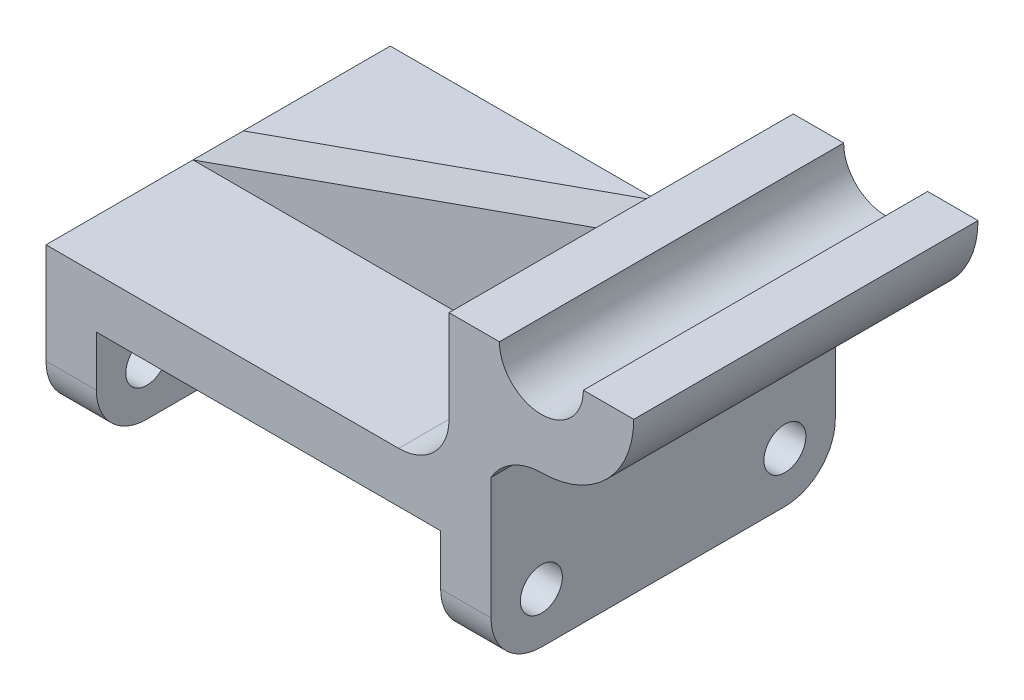
ISO-10303-21;
HEADER;
FILE_DESCRIPTION(('STEP AP214'),'2;1');
FILE_NAME('part.step','',(''),(''),'','','');
FILE_SCHEMA(('AUTOMOTIVE_DESIGN { 1 0 10303 214 1 1 1 1 }'));
ENDSEC;
DATA;
#1=APPLICATION_CONTEXT('core data for automotive mechanical design processes');
#2=APPLICATION_PROTOCOL_DEFINITION('international standard','automotive_design',2000,#1);
#3=PRODUCT_CONTEXT('',#1,'mechanical');
#4=PRODUCT('Part','Part','',(#3));
#5=PRODUCT_RELATED_PRODUCT_CATEGORY('part','',(#4));
#6=PRODUCT_DEFINITION_FORMATION('','',#4);
#7=PRODUCT_DEFINITION_CONTEXT('part definition',#1,'design');
#8=PRODUCT_DEFINITION('design','',#6,#7);
#9=PRODUCT_DEFINITION_SHAPE('','',#8);
#10=(LENGTH_UNIT() NAMED_UNIT(*) SI_UNIT(.MILLI.,.METRE.));
#11=(NAMED_UNIT(*) PLANE_ANGLE_UNIT() SI_UNIT($,.RADIAN.));
#12=(NAMED_UNIT(*) SI_UNIT($,.STERADIAN.) SOLID_ANGLE_UNIT());
#13=UNCERTAINTY_MEASURE_WITH_UNIT(LENGTH_MEASURE(1.E-05),#10,'distance_accuracy_value','');
#14=(GEOMETRIC_REPRESENTATION_CONTEXT(3) GLOBAL_UNCERTAINTY_ASSIGNED_CONTEXT((#13)) GLOBAL_UNIT_ASSIGNED_CONTEXT((#10,
#11,#12)) REPRESENTATION_CONTEXT('',''));
#15=CARTESIAN_POINT('',(0.,0.,0.));
#16=DIRECTION('',(0.,0.,1.));
#17=DIRECTION('',(1.,0.,0.));
#18=AXIS2_PLACEMENT_3D('',#15,#16,#17);
#19=CARTESIAN_POINT('',(0.,12.,0.));
#20=DIRECTION('',(0.,-1.,0.));
#21=DIRECTION('',(0.,0.,-1.));
#22=AXIS2_PLACEMENT_3D('',#19,#20,#21);
#23=PLANE('',#22);
#24=DIRECTION('',(1.,0.,0.));
#25=VECTOR('',#24,1.);
#26=CARTESIAN_POINT('',(-53.,12.,6.));
#27=LINE('',#26,#25);
#28=CARTESIAN_POINT('',(-53.,12.,6.));
#29=VERTEX_POINT('',#28);
#30=CARTESIAN_POINT('',(31.0000000000001,12.,6.));
#31=VERTEX_POINT('',#30);
#32=EDGE_CURVE('E380',#29,#31,#27,.T.);
#33=ORIENTED_EDGE('',*,*,#32,.F.);
#34=DIRECTION('',(0.,0.,1.));
#35=VECTOR('',#34,1.);
#36=CARTESIAN_POINT('',(-53.,12.,41.));
#37=LINE('',#36,#35);
#38=CARTESIAN_POINT('',(-53.,12.,41.));
#39=VERTEX_POINT('',#38);
#40=EDGE_CURVE('E368',#29,#39,#37,.T.);
#41=ORIENTED_EDGE('',*,*,#40,.T.);
#42=DIRECTION('',(1.,0.,0.));
#43=VECTOR('',#42,1.);
#44=CARTESIAN_POINT('',(-53.,12.,41.));
#45=LINE('',#44,#43);
#46=CARTESIAN_POINT('',(31.,12.,41.));
#47=VERTEX_POINT('',#46);
#48=EDGE_CURVE('E319',#39,#47,#45,.T.);
#49=ORIENTED_EDGE('',*,*,#48,.T.);
#50=DIRECTION('',(0.,0.,1.));
#51=VECTOR('',#50,1.);
#52=CARTESIAN_POINT('',(31.,12.,0.));
#53=LINE('',#52,#51);
#54=EDGE_CURVE('E230',#47,#31,#53,.F.);
#55=ORIENTED_EDGE('',*,*,#54,.T.);
#56=EDGE_LOOP('',(#33,#41,#49,#55));
#57=FACE_BOUND('',#56,.T.);
#58=ADVANCED_FACE('F39',(#57),#23,.F.);
#59=CARTESIAN_POINT('',(43.,12.,-41.));
#60=DIRECTION('',(-1.,0.,0.));
#61=DIRECTION('',(0.,0.,1.));
#62=AXIS2_PLACEMENT_3D('',#59,#60,#61);
#63=PLANE('',#62);
#64=DIRECTION('',(0.,0.,1.));
#65=VECTOR('',#64,1.);
#66=CARTESIAN_POINT('',(43.,46.,-41.));
#67=LINE('',#66,#65);
#68=CARTESIAN_POINT('',(43.,46.,6.));
#69=VERTEX_POINT('',#68);
#70=CARTESIAN_POINT('',(43.,46.,41.));
#71=VERTEX_POINT('',#70);
#72=EDGE_CURVE('E314',#69,#71,#67,.T.);
#73=ORIENTED_EDGE('',*,*,#72,.F.);
#74=DIRECTION('',(0.,1.,0.));
#75=VECTOR('',#74,1.);
#76=CARTESIAN_POINT('',(43.,46.,6.));
#77=LINE('',#76,#75);
#78=CARTESIAN_POINT('',(43.,24.,6.));
#79=VERTEX_POINT('',#78);
#80=EDGE_CURVE('E386',#79,#69,#77,.T.);
#81=ORIENTED_EDGE('',*,*,#80,.F.);
#82=DIRECTION('',(0.,0.,1.));
#83=VECTOR('',#82,1.);
#84=CARTESIAN_POINT('',(43.,24.,-41.));
#85=LINE('',#84,#83);
#86=CARTESIAN_POINT('',(43.,24.,41.));
#87=VERTEX_POINT('',#86);
#88=EDGE_CURVE('E220',#79,#87,#85,.T.);
#89=ORIENTED_EDGE('',*,*,#88,.T.);
#90=DIRECTION('',(0.,-1.,0.));
#91=VECTOR('',#90,1.);
#92=CARTESIAN_POINT('',(43.,12.,41.));
#93=LINE('',#92,#91);
#94=EDGE_CURVE('E363',#71,#87,#93,.T.);
#95=ORIENTED_EDGE('',*,*,#94,.F.);
#96=EDGE_LOOP('',(#73,#81,#89,#95));
#97=FACE_BOUND('',#96,.T.);
#98=ADVANCED_FACE('F427',(#97),#63,.T.);
#99=CARTESIAN_POINT('',(31.,24.,-41.));
#100=DIRECTION('',(0.,0.,1.));
#101=DIRECTION('',(1.,0.,0.));
#102=AXIS2_PLACEMENT_3D('',#99,#100,#101);
#103=CYLINDRICAL_SURFACE('',#102,12.);
#104=CARTESIAN_POINT('',(30.9999999999986,24.0000000000014,6.));
#105=DIRECTION('',(0.,0.,1.));
#106=DIRECTION('',(-1.,0.,0.));
#107=AXIS2_PLACEMENT_3D('',#104,#105,#106);
#108=CIRCLE('',#107,12.0000000000014);
#109=EDGE_CURVE('E510',#31,#79,#108,.T.);
#110=ORIENTED_EDGE('',*,*,#109,.F.);
#111=ORIENTED_EDGE('',*,*,#54,.F.);
#112=CARTESIAN_POINT('',(31.,24.,41.));
#113=DIRECTION('',(0.,0.,-1.));
#114=DIRECTION('',(-1.,0.,0.));
#115=AXIS2_PLACEMENT_3D('',#112,#113,#114);
#116=CIRCLE('',#115,12.);
#117=EDGE_CURVE('E235',#87,#47,#116,.T.);
#118=ORIENTED_EDGE('',*,*,#117,.F.);
#119=ORIENTED_EDGE('',*,*,#88,.F.);
#120=EDGE_LOOP('',(#110,#111,#118,#119));
#121=FACE_BOUND('',#120,.T.);
#122=ADVANCED_FACE('F440',(#121),#103,.F.);
#123=CARTESIAN_POINT('',(0.,0.,0.));
#124=DIRECTION('',(0.,-1.,0.));
#125=DIRECTION('',(0.,0.,-1.));
#126=AXIS2_PLACEMENT_3D('',#123,#124,#125);
#127=PLANE('',#126);
#128=DIRECTION('',(-1.,0.,0.));
#129=VECTOR('',#128,1.);
#130=CARTESIAN_POINT('',(-53.,0.,-41.));
#131=LINE('',#130,#129);
#132=CARTESIAN_POINT('',(41.,0.,-41.));
#133=VERTEX_POINT('',#132);
#134=CARTESIAN_POINT('',(-41.,0.,-41.));
#135=VERTEX_POINT('',#134);
#136=EDGE_CURVE('E295',#133,#135,#131,.T.);
#137=ORIENTED_EDGE('',*,*,#136,.F.);
#138=DIRECTION('',(0.,0.,1.));
#139=VECTOR('',#138,1.);
#140=CARTESIAN_POINT('',(41.,0.,41.));
#141=LINE('',#140,#139);
#142=CARTESIAN_POINT('',(41.,0.,41.));
#143=VERTEX_POINT('',#142);
#144=EDGE_CURVE('E298',#133,#143,#141,.T.);
#145=ORIENTED_EDGE('',*,*,#144,.T.);
#146=DIRECTION('',(1.,0.,0.));
#147=VECTOR('',#146,1.);
#148=CARTESIAN_POINT('',(-53.,0.,41.));
#149=LINE('',#148,#147);
#150=CARTESIAN_POINT('',(-41.,0.,41.));
#151=VERTEX_POINT('',#150);
#152=EDGE_CURVE('E307',#151,#143,#149,.T.);
#153=ORIENTED_EDGE('',*,*,#152,.F.);
#154=DIRECTION('',(0.,0.,-1.));
#155=VECTOR('',#154,1.);
#156=CARTESIAN_POINT('',(-41.,0.,-41.));
#157=LINE('',#156,#155);
#158=EDGE_CURVE('E308',#151,#135,#157,.T.);
#159=ORIENTED_EDGE('',*,*,#158,.T.);
#160=EDGE_LOOP('',(#137,#145,#153,#159));
#161=FACE_BOUND('',#160,.T.);
#162=ADVANCED_FACE('F306',(#161),#127,.T.);
#163=CARTESIAN_POINT('',(-53.,12.,-41.));
#164=VERTEX_POINT('',#163);
#165=CARTESIAN_POINT('',(-53.,12.,-6.));
#166=VERTEX_POINT('',#165);
#167=EDGE_CURVE('E367',#164,#166,#37,.T.);
#168=ORIENTED_EDGE('',*,*,#167,.T.);
#169=DIRECTION('',(1.,0.,0.));
#170=VECTOR('',#169,1.);
#171=CARTESIAN_POINT('',(-53.,12.,-6.));
#172=LINE('',#171,#170);
#173=CARTESIAN_POINT('',(31.0000000000001,12.,-6.));
#174=VERTEX_POINT('',#173);
#175=EDGE_CURVE('E480',#166,#174,#172,.T.);
#176=ORIENTED_EDGE('',*,*,#175,.T.);
#177=CARTESIAN_POINT('',(31.,12.,-41.));
#178=VERTEX_POINT('',#177);
#179=EDGE_CURVE('E226',#174,#178,#53,.F.);
#180=ORIENTED_EDGE('',*,*,#179,.T.);
#181=DIRECTION('',(-1.,0.,0.));
#182=VECTOR('',#181,1.);
#183=CARTESIAN_POINT('',(-53.,12.,-41.));
#184=LINE('',#183,#182);
#185=EDGE_CURVE('E315',#178,#164,#184,.T.);
#186=ORIENTED_EDGE('',*,*,#185,.T.);
#187=EDGE_LOOP('',(#168,#176,#180,#186));
#188=FACE_BOUND('',#187,.T.);
#189=ADVANCED_FACE('F435',(#188),#23,.F.);
#190=CARTESIAN_POINT('',(53.,12.,41.));
#191=DIRECTION('',(-1.,0.,0.));
#192=DIRECTION('',(0.,0.,1.));
#193=AXIS2_PLACEMENT_3D('',#190,#191,#192);
#194=PLANE('',#193);
#195=CARTESIAN_POINT('',(53.,-12.,29.));
#196=DIRECTION('',(1.,0.,0.));
#197=DIRECTION('',(0.,0.,-1.));
#198=AXIS2_PLACEMENT_3D('',#195,#196,#197);
#199=CIRCLE('',#198,5.);
#200=CARTESIAN_POINT('',(53.,-12.,24.));
#201=VERTEX_POINT('',#200);
#202=EDGE_CURVE('E396',#201,#201,#199,.T.);
#203=ORIENTED_EDGE('',*,*,#202,.F.);
#204=EDGE_LOOP('',(#203));
#205=FACE_BOUND('',#204,.T.);
#206=CARTESIAN_POINT('',(53.,-12.,-29.));
#207=DIRECTION('',(1.,0.,0.));
#208=DIRECTION('',(0.,0.,-1.));
#209=AXIS2_PLACEMENT_3D('',#206,#207,#208);
#210=CIRCLE('',#209,5.);
#211=CARTESIAN_POINT('',(53.,-12.,-34.));
#212=VERTEX_POINT('',#211);
#213=EDGE_CURVE('E390',#212,#212,#210,.T.);
#214=ORIENTED_EDGE('',*,*,#213,.F.);
#215=EDGE_LOOP('',(#214));
#216=FACE_BOUND('',#215,.T.);
#217=DIRECTION('',(0.,-1.,0.));
#218=VECTOR('',#217,1.);
#219=CARTESIAN_POINT('',(53.,12.,-41.));
#220=LINE('',#219,#218);
#221=CARTESIAN_POINT('',(53.,17.,-41.));
#222=VERTEX_POINT('',#221);
#223=CARTESIAN_POINT('',(53.,-12.,-41.));
#224=VERTEX_POINT('',#223);
#225=EDGE_CURVE('E207',#222,#224,#220,.T.);
#226=ORIENTED_EDGE('',*,*,#225,.F.);
#227=DIRECTION('',(0.,0.,1.));
#228=VECTOR('',#227,1.);
#229=CARTESIAN_POINT('',(53.,17.,-41.));
#230=LINE('',#229,#228);
#231=CARTESIAN_POINT('',(53.,17.,41.));
#232=VERTEX_POINT('',#231);
#233=EDGE_CURVE('E194',#222,#232,#230,.T.);
#234=ORIENTED_EDGE('',*,*,#233,.T.);
#235=DIRECTION('',(0.,-1.,0.));
#236=VECTOR('',#235,1.);
#237=CARTESIAN_POINT('',(53.,12.,41.));
#238=LINE('',#237,#236);
#239=CARTESIAN_POINT('',(53.,-12.,41.));
#240=VERTEX_POINT('',#239);
#241=EDGE_CURVE('E322',#232,#240,#238,.T.);
#242=ORIENTED_EDGE('',*,*,#241,.T.);
#243=CARTESIAN_POINT('',(53.,-12.,29.));
#244=DIRECTION('',(-1.,0.,0.));
#245=DIRECTION('',(0.,0.,1.));
#246=AXIS2_PLACEMENT_3D('',#243,#244,#245);
#247=CIRCLE('',#246,12.);
#248=CARTESIAN_POINT('',(53.,-24.,29.));
#249=VERTEX_POINT('',#248);
#250=EDGE_CURVE('E270',#240,#249,#247,.F.);
#251=ORIENTED_EDGE('',*,*,#250,.T.);
#252=DIRECTION('',(0.,0.,-1.));
#253=VECTOR('',#252,1.);
#254=CARTESIAN_POINT('',(53.,-24.,41.));
#255=LINE('',#254,#253);
#256=CARTESIAN_POINT('',(53.,-24.,-29.));
#257=VERTEX_POINT('',#256);
#258=EDGE_CURVE('E399',#249,#257,#255,.T.);
#259=ORIENTED_EDGE('',*,*,#258,.T.);
#260=CARTESIAN_POINT('',(53.,-12.,-29.));
#261=DIRECTION('',(-1.,0.,0.));
#262=DIRECTION('',(0.,0.,1.));
#263=AXIS2_PLACEMENT_3D('',#260,#261,#262);
#264=CIRCLE('',#263,12.);
#265=EDGE_CURVE('E213',#257,#224,#264,.F.);
#266=ORIENTED_EDGE('',*,*,#265,.T.);
#267=EDGE_LOOP('',(#226,#234,#242,#251,#259,#266));
#268=FACE_BOUND('',#267,.T.);
#269=ADVANCED_FACE('F214',(#205,#216,#268),#194,.F.);
#270=CARTESIAN_POINT('',(-53.,12.,-41.));
#271=DIRECTION('',(0.,0.,1.));
#272=DIRECTION('',(1.,0.,0.));
#273=AXIS2_PLACEMENT_3D('',#270,#271,#272);
#274=PLANE('',#273);
#275=DIRECTION('',(-1.,0.,0.));
#276=VECTOR('',#275,1.);
#277=CARTESIAN_POINT('',(53.,46.,-41.));
#278=LINE('',#277,#276);
#279=CARTESIAN_POINT('',(55.,46.,-41.));
#280=VERTEX_POINT('',#279);
#281=CARTESIAN_POINT('',(43.,46.,-41.));
#282=VERTEX_POINT('',#281);
#283=EDGE_CURVE('E357',#280,#282,#278,.T.);
#284=ORIENTED_EDGE('',*,*,#283,.F.);
#285=CARTESIAN_POINT('',(65.,46.,-41.));
#286=DIRECTION('',(0.,0.,-1.));
#287=DIRECTION('',(1.,0.,0.));
#288=AXIS2_PLACEMENT_3D('',#285,#286,#287);
#289=CIRCLE('',#288,10.);
#290=CARTESIAN_POINT('',(75.,46.,-41.));
#291=VERTEX_POINT('',#290);
#292=EDGE_CURVE('E202',#291,#280,#289,.T.);
#293=ORIENTED_EDGE('',*,*,#292,.F.);
#294=DIRECTION('',(-1.,0.,0.));
#295=VECTOR('',#294,1.);
#296=CARTESIAN_POINT('',(75.,46.,-41.));
#297=LINE('',#296,#295);
#298=CARTESIAN_POINT('',(87.,46.,-41.));
#299=VERTEX_POINT('',#298);
#300=EDGE_CURVE('E764',#299,#291,#297,.T.);
#301=ORIENTED_EDGE('',*,*,#300,.F.);
#302=CARTESIAN_POINT('',(65.,46.,-41.));
#303=DIRECTION('',(0.,0.,1.));
#304=DIRECTION('',(1.,0.,0.));
#305=AXIS2_PLACEMENT_3D('',#302,#303,#304);
#306=CIRCLE('',#305,22.);
#307=CARTESIAN_POINT('',(65.0760710520603,24.0001315186877,-41.));
#308=VERTEX_POINT('',#307);
#309=EDGE_CURVE('E208',#308,#299,#306,.T.);
#310=ORIENTED_EDGE('',*,*,#309,.F.);
#311=CARTESIAN_POINT('',(65.1244799033714,10.0002152123981,-41.));
#312=DIRECTION('',(0.,0.,-1.));
#313=DIRECTION('',(-1.,0.,0.));
#314=AXIS2_PLACEMENT_3D('',#311,#312,#313);
#315=CIRCLE('',#314,14.);
#316=EDGE_CURVE('E198',#222,#308,#315,.T.);
#317=ORIENTED_EDGE('',*,*,#316,.F.);
#318=ORIENTED_EDGE('',*,*,#225,.T.);
#319=DIRECTION('',(1.,0.,0.));
#320=VECTOR('',#319,1.);
#321=CARTESIAN_POINT('',(41.,-12.,-41.));
#322=LINE('',#321,#320);
#323=CARTESIAN_POINT('',(41.,-12.,-41.));
#324=VERTEX_POINT('',#323);
#325=EDGE_CURVE('E268',#224,#324,#322,.F.);
#326=ORIENTED_EDGE('',*,*,#325,.T.);
#327=DIRECTION('',(0.,1.,0.));
#328=VECTOR('',#327,1.);
#329=CARTESIAN_POINT('',(41.,0.,-41.));
#330=LINE('',#329,#328);
#331=EDGE_CURVE('E285',#324,#133,#330,.T.);
#332=ORIENTED_EDGE('',*,*,#331,.T.);
#333=ORIENTED_EDGE('',*,*,#136,.T.);
#334=DIRECTION('',(0.,-1.,0.));
#335=VECTOR('',#334,1.);
#336=CARTESIAN_POINT('',(-41.,0.,-41.));
#337=LINE('',#336,#335);
#338=CARTESIAN_POINT('',(-41.,-12.,-41.));
#339=VERTEX_POINT('',#338);
#340=EDGE_CURVE('E346',#135,#339,#337,.T.);
#341=ORIENTED_EDGE('',*,*,#340,.T.);
#342=DIRECTION('',(-1.,0.,0.));
#343=VECTOR('',#342,1.);
#344=CARTESIAN_POINT('',(-53.,-12.,-41.));
#345=LINE('',#344,#343);
#346=CARTESIAN_POINT('',(-53.,-12.,-41.));
#347=VERTEX_POINT('',#346);
#348=EDGE_CURVE('E236',#339,#347,#345,.T.);
#349=ORIENTED_EDGE('',*,*,#348,.T.);
#350=DIRECTION('',(0.,-1.,0.));
#351=VECTOR('',#350,1.);
#352=CARTESIAN_POINT('',(-53.,12.,-41.));
#353=LINE('',#352,#351);
#354=EDGE_CURVE('E216',#164,#347,#353,.T.);
#355=ORIENTED_EDGE('',*,*,#354,.F.);
#356=ORIENTED_EDGE('',*,*,#185,.F.);
#357=CARTESIAN_POINT('',(31.,24.,-41.));
#358=DIRECTION('',(0.,0.,1.));
#359=DIRECTION('',(1.,0.,0.));
#360=AXIS2_PLACEMENT_3D('',#357,#358,#359);
#361=CIRCLE('',#360,12.);
#362=CARTESIAN_POINT('',(43.,24.,-41.));
#363=VERTEX_POINT('',#362);
#364=EDGE_CURVE('E234',#178,#363,#361,.T.);
#365=ORIENTED_EDGE('',*,*,#364,.T.);
#366=DIRECTION('',(0.,-1.,0.));
#367=VECTOR('',#366,1.);
#368=CARTESIAN_POINT('',(43.,12.,-41.));
#369=LINE('',#368,#367);
#370=EDGE_CURVE('E359',#282,#363,#369,.T.);
#371=ORIENTED_EDGE('',*,*,#370,.F.);
#372=EDGE_LOOP('',(#284,#293,#301,#310,#317,#318,#326,#332,#333,#341,#349,#355,#356,#365,#371));
#373=FACE_BOUND('',#372,.T.);
#374=ADVANCED_FACE('F203',(#373),#274,.F.);
#375=CARTESIAN_POINT('',(-53.,12.,41.));
#376=DIRECTION('',(1.,0.,0.));
#377=DIRECTION('',(0.,0.,-1.));
#378=AXIS2_PLACEMENT_3D('',#375,#376,#377);
#379=PLANE('',#378);
#380=CARTESIAN_POINT('',(-53.,-12.,-29.));
#381=DIRECTION('',(-1.,0.,0.));
#382=DIRECTION('',(0.,0.,1.));
#383=AXIS2_PLACEMENT_3D('',#380,#381,#382);
#384=CIRCLE('',#383,5.);
#385=CARTESIAN_POINT('',(-53.,-12.,-24.));
#386=VERTEX_POINT('',#385);
#387=EDGE_CURVE('E256',#386,#386,#384,.T.);
#388=ORIENTED_EDGE('',*,*,#387,.F.);
#389=EDGE_LOOP('',(#388));
#390=FACE_BOUND('',#389,.T.);
#391=CARTESIAN_POINT('',(-53.,-12.,29.));
#392=DIRECTION('',(-1.,0.,0.));
#393=DIRECTION('',(0.,0.,1.));
#394=AXIS2_PLACEMENT_3D('',#391,#392,#393);
#395=CIRCLE('',#394,5.);
#396=CARTESIAN_POINT('',(-53.,-12.,34.));
#397=VERTEX_POINT('',#396);
#398=EDGE_CURVE('E303',#397,#397,#395,.T.);
#399=ORIENTED_EDGE('',*,*,#398,.F.);
#400=EDGE_LOOP('',(#399));
#401=FACE_BOUND('',#400,.T.);
#402=ORIENTED_EDGE('',*,*,#354,.T.);
#403=CARTESIAN_POINT('',(-53.,-12.,-29.));
#404=DIRECTION('',(1.,0.,0.));
#405=DIRECTION('',(0.,0.,-1.));
#406=AXIS2_PLACEMENT_3D('',#403,#404,#405);
#407=CIRCLE('',#406,12.);
#408=CARTESIAN_POINT('',(-53.,-24.,-29.));
#409=VERTEX_POINT('',#408);
#410=EDGE_CURVE('E241',#347,#409,#407,.F.);
#411=ORIENTED_EDGE('',*,*,#410,.T.);
#412=DIRECTION('',(0.,0.,1.));
#413=VECTOR('',#412,1.);
#414=CARTESIAN_POINT('',(-53.,-24.,-41.));
#415=LINE('',#414,#413);
#416=CARTESIAN_POINT('',(-53.,-24.,29.));
#417=VERTEX_POINT('',#416);
#418=EDGE_CURVE('E265',#409,#417,#415,.T.);
#419=ORIENTED_EDGE('',*,*,#418,.T.);
#420=CARTESIAN_POINT('',(-53.,-12.,29.));
#421=DIRECTION('',(1.,0.,0.));
#422=DIRECTION('',(0.,0.,-1.));
#423=AXIS2_PLACEMENT_3D('',#420,#421,#422);
#424=CIRCLE('',#423,12.);
#425=CARTESIAN_POINT('',(-53.,-12.,41.));
#426=VERTEX_POINT('',#425);
#427=EDGE_CURVE('E237',#417,#426,#424,.F.);
#428=ORIENTED_EDGE('',*,*,#427,.T.);
#429=DIRECTION('',(0.,-1.,0.));
#430=VECTOR('',#429,1.);
#431=CARTESIAN_POINT('',(-53.,12.,41.));
#432=LINE('',#431,#430);
#433=EDGE_CURVE('E224',#39,#426,#432,.T.);
#434=ORIENTED_EDGE('',*,*,#433,.F.);
#435=ORIENTED_EDGE('',*,*,#40,.F.);
#436=DIRECTION('',(0.,0.,-1.));
#437=VECTOR('',#436,1.);
#438=CARTESIAN_POINT('',(-53.,12.,6.));
#439=LINE('',#438,#437);
#440=EDGE_CURVE('E382',#29,#166,#439,.T.);
#441=ORIENTED_EDGE('',*,*,#440,.T.);
#442=ORIENTED_EDGE('',*,*,#167,.F.);
#443=EDGE_LOOP('',(#402,#411,#419,#428,#434,#435,#441,#442));
#444=FACE_BOUND('',#443,.T.);
#445=ADVANCED_FACE('F378',(#390,#401,#444),#379,.F.);
#446=CARTESIAN_POINT('',(-53.,12.,41.));
#447=DIRECTION('',(0.,0.,-1.));
#448=DIRECTION('',(-1.,0.,0.));
#449=AXIS2_PLACEMENT_3D('',#446,#447,#448);
#450=PLANE('',#449);
#451=DIRECTION('',(0.,-1.,0.));
#452=VECTOR('',#451,1.);
#453=CARTESIAN_POINT('',(41.,0.,41.));
#454=LINE('',#453,#452);
#455=CARTESIAN_POINT('',(41.,-12.,41.));
#456=VERTEX_POINT('',#455);
#457=EDGE_CURVE('E286',#143,#456,#454,.T.);
#458=ORIENTED_EDGE('',*,*,#457,.T.);
#459=DIRECTION('',(1.,0.,0.));
#460=VECTOR('',#459,1.);
#461=CARTESIAN_POINT('',(53.,-12.,41.));
#462=LINE('',#461,#460);
#463=EDGE_CURVE('E11',#456,#240,#462,.T.);
#464=ORIENTED_EDGE('',*,*,#463,.T.);
#465=ORIENTED_EDGE('',*,*,#241,.F.);
#466=CARTESIAN_POINT('',(65.1244799033714,10.0002152123981,41.));
#467=DIRECTION('',(0.,0.,-1.));
#468=DIRECTION('',(-1.,0.,0.));
#469=AXIS2_PLACEMENT_3D('',#466,#467,#468);
#470=CIRCLE('',#469,14.);
#471=CARTESIAN_POINT('',(65.0760710520603,24.0001315186877,41.));
#472=VERTEX_POINT('',#471);
#473=EDGE_CURVE('E53',#232,#472,#470,.T.);
#474=ORIENTED_EDGE('',*,*,#473,.T.);
#475=CARTESIAN_POINT('',(65.,46.,41.));
#476=DIRECTION('',(0.,0.,1.));
#477=DIRECTION('',(1.,0.,0.));
#478=AXIS2_PLACEMENT_3D('',#475,#476,#477);
#479=CIRCLE('',#478,22.);
#480=CARTESIAN_POINT('',(87.,46.,41.));
#481=VERTEX_POINT('',#480);
#482=EDGE_CURVE('E486',#472,#481,#479,.T.);
#483=ORIENTED_EDGE('',*,*,#482,.T.);
#484=DIRECTION('',(-1.,0.,0.));
#485=VECTOR('',#484,1.);
#486=CARTESIAN_POINT('',(75.,46.,41.));
#487=LINE('',#486,#485);
#488=CARTESIAN_POINT('',(75.,46.,41.));
#489=VERTEX_POINT('',#488);
#490=EDGE_CURVE('E489',#481,#489,#487,.T.);
#491=ORIENTED_EDGE('',*,*,#490,.T.);
#492=CARTESIAN_POINT('',(65.,46.,41.));
#493=DIRECTION('',(0.,0.,-1.));
#494=DIRECTION('',(1.,0.,0.));
#495=AXIS2_PLACEMENT_3D('',#492,#493,#494);
#496=CIRCLE('',#495,10.);
#497=CARTESIAN_POINT('',(55.,46.,41.));
#498=VERTEX_POINT('',#497);
#499=EDGE_CURVE('E212',#489,#498,#496,.T.);
#500=ORIENTED_EDGE('',*,*,#499,.T.);
#501=DIRECTION('',(-1.,0.,0.));
#502=VECTOR('',#501,1.);
#503=CARTESIAN_POINT('',(53.,46.,41.));
#504=LINE('',#503,#502);
#505=EDGE_CURVE('E353',#498,#71,#504,.T.);
#506=ORIENTED_EDGE('',*,*,#505,.T.);
#507=ORIENTED_EDGE('',*,*,#94,.T.);
#508=ORIENTED_EDGE('',*,*,#117,.T.);
#509=ORIENTED_EDGE('',*,*,#48,.F.);
#510=ORIENTED_EDGE('',*,*,#433,.T.);
#511=DIRECTION('',(-1.,0.,0.));
#512=VECTOR('',#511,1.);
#513=CARTESIAN_POINT('',(-41.,-12.,41.));
#514=LINE('',#513,#512);
#515=CARTESIAN_POINT('',(-41.,-12.,41.));
#516=VERTEX_POINT('',#515);
#517=EDGE_CURVE('E255',#426,#516,#514,.F.);
#518=ORIENTED_EDGE('',*,*,#517,.T.);
#519=DIRECTION('',(0.,1.,0.));
#520=VECTOR('',#519,1.);
#521=CARTESIAN_POINT('',(-41.,0.,41.));
#522=LINE('',#521,#520);
#523=EDGE_CURVE('E345',#516,#151,#522,.T.);
#524=ORIENTED_EDGE('',*,*,#523,.T.);
#525=ORIENTED_EDGE('',*,*,#152,.T.);
#526=EDGE_LOOP('',(#458,#464,#465,#474,#483,#491,#500,#506,#507,#508,#509,#510,#518,#524,#525));
#527=FACE_BOUND('',#526,.T.);
#528=ADVANCED_FACE('F330',(#527),#450,.F.);
#529=DIRECTION('',(0.,1.,0.));
#530=VECTOR('',#529,1.);
#531=CARTESIAN_POINT('',(43.,46.,-6.));
#532=LINE('',#531,#530);
#533=CARTESIAN_POINT('',(43.,24.,-6.));
#534=VERTEX_POINT('',#533);
#535=CARTESIAN_POINT('',(43.,46.,-6.));
#536=VERTEX_POINT('',#535);
#537=EDGE_CURVE('E65',#534,#536,#532,.T.);
#538=ORIENTED_EDGE('',*,*,#537,.T.);
#539=EDGE_CURVE('E309',#282,#536,#67,.T.);
#540=ORIENTED_EDGE('',*,*,#539,.F.);
#541=ORIENTED_EDGE('',*,*,#370,.T.);
#542=EDGE_CURVE('E219',#363,#534,#85,.T.);
#543=ORIENTED_EDGE('',*,*,#542,.T.);
#544=EDGE_LOOP('',(#538,#540,#541,#543));
#545=FACE_BOUND('',#544,.T.);
#546=ADVANCED_FACE('F425',(#545),#63,.T.);
#547=CARTESIAN_POINT('',(53.,46.,-41.));
#548=DIRECTION('',(0.,1.,0.));
#549=DIRECTION('',(0.,0.,1.));
#550=AXIS2_PLACEMENT_3D('',#547,#548,#549);
#551=PLANE('',#550);
#552=ORIENTED_EDGE('',*,*,#505,.F.);
#553=DIRECTION('',(0.,0.,1.));
#554=VECTOR('',#553,1.);
#555=CARTESIAN_POINT('',(55.,46.,-41.));
#556=LINE('',#555,#554);
#557=EDGE_CURVE('E498',#280,#498,#556,.T.);
#558=ORIENTED_EDGE('',*,*,#557,.F.);
#559=ORIENTED_EDGE('',*,*,#283,.T.);
#560=ORIENTED_EDGE('',*,*,#539,.T.);
#561=DIRECTION('',(0.,0.,-1.));
#562=VECTOR('',#561,1.);
#563=CARTESIAN_POINT('',(43.,46.,6.));
#564=LINE('',#563,#562);
#565=EDGE_CURVE('E381',#69,#536,#564,.T.);
#566=ORIENTED_EDGE('',*,*,#565,.F.);
#567=ORIENTED_EDGE('',*,*,#72,.T.);
#568=EDGE_LOOP('',(#552,#558,#559,#560,#566,#567));
#569=FACE_BOUND('',#568,.T.);
#570=ADVANCED_FACE('F462',(#569),#551,.T.);
#571=ORIENTED_EDGE('',*,*,#179,.F.);
#572=CARTESIAN_POINT('',(30.9999999999986,24.0000000000014,-6.));
#573=DIRECTION('',(0.,0.,1.));
#574=DIRECTION('',(-1.,0.,0.));
#575=AXIS2_PLACEMENT_3D('',#572,#573,#574);
#576=CIRCLE('',#575,12.0000000000014);
#577=EDGE_CURVE('E474',#174,#534,#576,.T.);
#578=ORIENTED_EDGE('',*,*,#577,.T.);
#579=ORIENTED_EDGE('',*,*,#542,.F.);
#580=ORIENTED_EDGE('',*,*,#364,.F.);
#581=EDGE_LOOP('',(#571,#578,#579,#580));
#582=FACE_BOUND('',#581,.T.);
#583=ADVANCED_FACE('F453',(#582),#103,.F.);
#584=CARTESIAN_POINT('',(-41.,-24.,-41.));
#585=DIRECTION('',(0.,-1.,0.));
#586=DIRECTION('',(0.,0.,-1.));
#587=AXIS2_PLACEMENT_3D('',#584,#585,#586);
#588=PLANE('',#587);
#589=ORIENTED_EDGE('',*,*,#418,.F.);
#590=DIRECTION('',(-1.,0.,0.));
#591=VECTOR('',#590,1.);
#592=CARTESIAN_POINT('',(-41.,-24.,-29.));
#593=LINE('',#592,#591);
#594=CARTESIAN_POINT('',(-41.,-24.,-29.));
#595=VERTEX_POINT('',#594);
#596=EDGE_CURVE('E246',#409,#595,#593,.F.);
#597=ORIENTED_EDGE('',*,*,#596,.T.);
#598=DIRECTION('',(0.,0.,1.));
#599=VECTOR('',#598,1.);
#600=CARTESIAN_POINT('',(-41.,-24.,-41.));
#601=LINE('',#600,#599);
#602=CARTESIAN_POINT('',(-41.,-24.,29.));
#603=VERTEX_POINT('',#602);
#604=EDGE_CURVE('E338',#595,#603,#601,.T.);
#605=ORIENTED_EDGE('',*,*,#604,.T.);
#606=DIRECTION('',(-1.,0.,0.));
#607=VECTOR('',#606,1.);
#608=CARTESIAN_POINT('',(-53.,-24.,29.));
#609=LINE('',#608,#607);
#610=EDGE_CURVE('E243',#603,#417,#609,.T.);
#611=ORIENTED_EDGE('',*,*,#610,.T.);
#612=EDGE_LOOP('',(#589,#597,#605,#611));
#613=FACE_BOUND('',#612,.T.);
#614=ADVANCED_FACE('F343',(#613),#588,.T.);
#615=CARTESIAN_POINT('',(-41.,0.,0.));
#616=DIRECTION('',(-1.,0.,0.));
#617=DIRECTION('',(0.,0.,1.));
#618=AXIS2_PLACEMENT_3D('',#615,#616,#617);
#619=PLANE('',#618);
#620=CARTESIAN_POINT('',(-41.,-12.,-29.));
#621=DIRECTION('',(-1.,0.,0.));
#622=DIRECTION('',(0.,0.,1.));
#623=AXIS2_PLACEMENT_3D('',#620,#621,#622);
#624=CIRCLE('',#623,5.);
#625=CARTESIAN_POINT('',(-41.,-12.,-24.));
#626=VERTEX_POINT('',#625);
#627=EDGE_CURVE('E259',#626,#626,#624,.T.);
#628=ORIENTED_EDGE('',*,*,#627,.T.);
#629=EDGE_LOOP('',(#628));
#630=FACE_BOUND('',#629,.T.);
#631=CARTESIAN_POINT('',(-41.,-12.,29.));
#632=DIRECTION('',(-1.,0.,0.));
#633=DIRECTION('',(0.,0.,1.));
#634=AXIS2_PLACEMENT_3D('',#631,#632,#633);
#635=CIRCLE('',#634,5.);
#636=CARTESIAN_POINT('',(-41.,-12.,34.));
#637=VERTEX_POINT('',#636);
#638=EDGE_CURVE('E253',#637,#637,#635,.T.);
#639=ORIENTED_EDGE('',*,*,#638,.T.);
#640=EDGE_LOOP('',(#639));
#641=FACE_BOUND('',#640,.T.);
#642=ORIENTED_EDGE('',*,*,#604,.F.);
#643=CARTESIAN_POINT('',(-41.,-12.,-29.));
#644=DIRECTION('',(-1.,0.,0.));
#645=DIRECTION('',(0.,0.,1.));
#646=AXIS2_PLACEMENT_3D('',#643,#644,#645);
#647=CIRCLE('',#646,12.);
#648=EDGE_CURVE('E249',#595,#339,#647,.F.);
#649=ORIENTED_EDGE('',*,*,#648,.T.);
#650=ORIENTED_EDGE('',*,*,#340,.F.);
#651=ORIENTED_EDGE('',*,*,#158,.F.);
#652=ORIENTED_EDGE('',*,*,#523,.F.);
#653=CARTESIAN_POINT('',(-41.,-12.,29.));
#654=DIRECTION('',(-1.,0.,0.));
#655=DIRECTION('',(0.,0.,1.));
#656=AXIS2_PLACEMENT_3D('',#653,#654,#655);
#657=CIRCLE('',#656,12.);
#658=EDGE_CURVE('E247',#516,#603,#657,.F.);
#659=ORIENTED_EDGE('',*,*,#658,.T.);
#660=EDGE_LOOP('',(#642,#649,#650,#651,#652,#659));
#661=FACE_BOUND('',#660,.T.);
#662=ADVANCED_FACE('F339',(#630,#641,#661),#619,.F.);
#663=CARTESIAN_POINT('',(-53.,-12.,-29.));
#664=DIRECTION('',(1.,0.,0.));
#665=DIRECTION('',(0.,0.,-1.));
#666=AXIS2_PLACEMENT_3D('',#663,#664,#665);
#667=CYLINDRICAL_SURFACE('',#666,12.);
#668=ORIENTED_EDGE('',*,*,#648,.F.);
#669=ORIENTED_EDGE('',*,*,#596,.F.);
#670=ORIENTED_EDGE('',*,*,#410,.F.);
#671=ORIENTED_EDGE('',*,*,#348,.F.);
#672=EDGE_LOOP('',(#668,#669,#670,#671));
#673=FACE_BOUND('',#672,.T.);
#674=ADVANCED_FACE('F482',(#673),#667,.T.);
#675=CARTESIAN_POINT('',(-41.,-12.,29.));
#676=DIRECTION('',(1.,0.,0.));
#677=DIRECTION('',(0.,0.,-1.));
#678=AXIS2_PLACEMENT_3D('',#675,#676,#677);
#679=CYLINDRICAL_SURFACE('',#678,12.);
#680=ORIENTED_EDGE('',*,*,#658,.F.);
#681=ORIENTED_EDGE('',*,*,#517,.F.);
#682=ORIENTED_EDGE('',*,*,#427,.F.);
#683=ORIENTED_EDGE('',*,*,#610,.F.);
#684=EDGE_LOOP('',(#680,#681,#682,#683));
#685=FACE_BOUND('',#684,.T.);
#686=ADVANCED_FACE('F331',(#685),#679,.T.);
#687=CARTESIAN_POINT('',(53.,-12.,29.));
#688=DIRECTION('',(-1.,0.,0.));
#689=DIRECTION('',(0.,0.,1.));
#690=AXIS2_PLACEMENT_3D('',#687,#688,#689);
#691=CYLINDRICAL_SURFACE('',#690,5.);
#692=ORIENTED_EDGE('',*,*,#398,.T.);
#693=EDGE_LOOP('',(#692));
#694=FACE_BOUND('',#693,.T.);
#695=ORIENTED_EDGE('',*,*,#638,.F.);
#696=EDGE_LOOP('',(#695));
#697=FACE_BOUND('',#696,.T.);
#698=ADVANCED_FACE('F411',(#694,#697),#691,.F.);
#699=CARTESIAN_POINT('',(53.,-12.,-29.));
#700=DIRECTION('',(-1.,0.,0.));
#701=DIRECTION('',(0.,0.,1.));
#702=AXIS2_PLACEMENT_3D('',#699,#700,#701);
#703=CYLINDRICAL_SURFACE('',#702,5.);
#704=ORIENTED_EDGE('',*,*,#387,.T.);
#705=EDGE_LOOP('',(#704));
#706=FACE_BOUND('',#705,.T.);
#707=ORIENTED_EDGE('',*,*,#627,.F.);
#708=EDGE_LOOP('',(#707));
#709=FACE_BOUND('',#708,.T.);
#710=ADVANCED_FACE('F545',(#706,#709),#703,.F.);
#711=CARTESIAN_POINT('',(41.,-24.,41.));
#712=DIRECTION('',(0.,-1.,0.));
#713=DIRECTION('',(0.,0.,-1.));
#714=AXIS2_PLACEMENT_3D('',#711,#712,#713);
#715=PLANE('',#714);
#716=DIRECTION('',(0.,0.,-1.));
#717=VECTOR('',#716,1.);
#718=CARTESIAN_POINT('',(41.,-24.,41.));
#719=LINE('',#718,#717);
#720=CARTESIAN_POINT('',(41.,-24.,29.));
#721=VERTEX_POINT('',#720);
#722=CARTESIAN_POINT('',(41.,-24.,-29.));
#723=VERTEX_POINT('',#722);
#724=EDGE_CURVE('E276',#721,#723,#719,.T.);
#725=ORIENTED_EDGE('',*,*,#724,.T.);
#726=DIRECTION('',(1.,0.,0.));
#727=VECTOR('',#726,1.);
#728=CARTESIAN_POINT('',(53.,-24.,-29.));
#729=LINE('',#728,#727);
#730=EDGE_CURVE('E262',#723,#257,#729,.T.);
#731=ORIENTED_EDGE('',*,*,#730,.T.);
#732=ORIENTED_EDGE('',*,*,#258,.F.);
#733=DIRECTION('',(1.,0.,0.));
#734=VECTOR('',#733,1.);
#735=CARTESIAN_POINT('',(41.,-24.,29.));
#736=LINE('',#735,#734);
#737=EDGE_CURVE('E251',#249,#721,#736,.F.);
#738=ORIENTED_EDGE('',*,*,#737,.T.);
#739=EDGE_LOOP('',(#725,#731,#732,#738));
#740=FACE_BOUND('',#739,.T.);
#741=ADVANCED_FACE('F287',(#740),#715,.T.);
#742=CARTESIAN_POINT('',(41.,0.,0.));
#743=DIRECTION('',(1.,0.,0.));
#744=DIRECTION('',(0.,0.,-1.));
#745=AXIS2_PLACEMENT_3D('',#742,#743,#744);
#746=PLANE('',#745);
#747=CARTESIAN_POINT('',(41.,-12.,29.));
#748=DIRECTION('',(1.,0.,0.));
#749=DIRECTION('',(0.,0.,-1.));
#750=AXIS2_PLACEMENT_3D('',#747,#748,#749);
#751=CIRCLE('',#750,5.);
#752=CARTESIAN_POINT('',(41.,-12.,24.));
#753=VERTEX_POINT('',#752);
#754=EDGE_CURVE('E394',#753,#753,#751,.T.);
#755=ORIENTED_EDGE('',*,*,#754,.T.);
#756=EDGE_LOOP('',(#755));
#757=FACE_BOUND('',#756,.T.);
#758=CARTESIAN_POINT('',(41.,-12.,-29.));
#759=DIRECTION('',(1.,0.,0.));
#760=DIRECTION('',(0.,0.,-1.));
#761=AXIS2_PLACEMENT_3D('',#758,#759,#760);
#762=CIRCLE('',#761,5.);
#763=CARTESIAN_POINT('',(41.,-12.,-34.));
#764=VERTEX_POINT('',#763);
#765=EDGE_CURVE('E405',#764,#764,#762,.T.);
#766=ORIENTED_EDGE('',*,*,#765,.T.);
#767=EDGE_LOOP('',(#766));
#768=FACE_BOUND('',#767,.T.);
#769=ORIENTED_EDGE('',*,*,#331,.F.);
#770=CARTESIAN_POINT('',(41.,-12.,-29.));
#771=DIRECTION('',(1.,0.,0.));
#772=DIRECTION('',(0.,0.,-1.));
#773=AXIS2_PLACEMENT_3D('',#770,#771,#772);
#774=CIRCLE('',#773,12.);
#775=EDGE_CURVE('E50',#324,#723,#774,.F.);
#776=ORIENTED_EDGE('',*,*,#775,.T.);
#777=ORIENTED_EDGE('',*,*,#724,.F.);
#778=CARTESIAN_POINT('',(41.,-12.,29.));
#779=DIRECTION('',(1.,0.,0.));
#780=DIRECTION('',(0.,0.,-1.));
#781=AXIS2_PLACEMENT_3D('',#778,#779,#780);
#782=CIRCLE('',#781,12.);
#783=EDGE_CURVE('E275',#721,#456,#782,.F.);
#784=ORIENTED_EDGE('',*,*,#783,.T.);
#785=ORIENTED_EDGE('',*,*,#457,.F.);
#786=ORIENTED_EDGE('',*,*,#144,.F.);
#787=EDGE_LOOP('',(#769,#776,#777,#784,#785,#786));
#788=FACE_BOUND('',#787,.T.);
#789=ADVANCED_FACE('F279',(#757,#768,#788),#746,.F.);
#790=CARTESIAN_POINT('',(41.,-12.,-29.));
#791=DIRECTION('',(-1.,0.,0.));
#792=DIRECTION('',(0.,0.,1.));
#793=AXIS2_PLACEMENT_3D('',#790,#791,#792);
#794=CYLINDRICAL_SURFACE('',#793,12.);
#795=ORIENTED_EDGE('',*,*,#775,.F.);
#796=ORIENTED_EDGE('',*,*,#325,.F.);
#797=ORIENTED_EDGE('',*,*,#265,.F.);
#798=ORIENTED_EDGE('',*,*,#730,.F.);
#799=EDGE_LOOP('',(#795,#796,#797,#798));
#800=FACE_BOUND('',#799,.T.);
#801=ADVANCED_FACE('F293',(#800),#794,.T.);
#802=CARTESIAN_POINT('',(-53.,-12.,29.));
#803=DIRECTION('',(-1.,0.,0.));
#804=DIRECTION('',(0.,0.,1.));
#805=AXIS2_PLACEMENT_3D('',#802,#803,#804);
#806=CYLINDRICAL_SURFACE('',#805,12.);
#807=ORIENTED_EDGE('',*,*,#783,.F.);
#808=ORIENTED_EDGE('',*,*,#737,.F.);
#809=ORIENTED_EDGE('',*,*,#250,.F.);
#810=ORIENTED_EDGE('',*,*,#463,.F.);
#811=EDGE_LOOP('',(#807,#808,#809,#810));
#812=FACE_BOUND('',#811,.T.);
#813=ADVANCED_FACE('F41',(#812),#806,.T.);
#814=CARTESIAN_POINT('',(41.,-12.,-29.));
#815=DIRECTION('',(1.,0.,0.));
#816=DIRECTION('',(0.,0.,-1.));
#817=AXIS2_PLACEMENT_3D('',#814,#815,#816);
#818=CYLINDRICAL_SURFACE('',#817,5.);
#819=ORIENTED_EDGE('',*,*,#765,.F.);
#820=EDGE_LOOP('',(#819));
#821=FACE_BOUND('',#820,.T.);
#822=ORIENTED_EDGE('',*,*,#213,.T.);
#823=EDGE_LOOP('',(#822));
#824=FACE_BOUND('',#823,.T.);
#825=ADVANCED_FACE('F531',(#821,#824),#818,.F.);
#826=CARTESIAN_POINT('',(41.,-12.,29.));
#827=DIRECTION('',(1.,0.,0.));
#828=DIRECTION('',(0.,0.,-1.));
#829=AXIS2_PLACEMENT_3D('',#826,#827,#828);
#830=CYLINDRICAL_SURFACE('',#829,5.);
#831=ORIENTED_EDGE('',*,*,#754,.F.);
#832=EDGE_LOOP('',(#831));
#833=FACE_BOUND('',#832,.T.);
#834=ORIENTED_EDGE('',*,*,#202,.T.);
#835=EDGE_LOOP('',(#834));
#836=FACE_BOUND('',#835,.T.);
#837=ADVANCED_FACE('F532',(#833,#836),#830,.F.);
#838=CARTESIAN_POINT('',(-53.,12.,6.));
#839=DIRECTION('',(0.333847142244594,-0.942627225161207,0.));
#840=DIRECTION('',(0.942627225161207,0.333847142244594,0.));
#841=AXIS2_PLACEMENT_3D('',#838,#839,#840);
#842=PLANE('',#841);
#843=DIRECTION('',(-0.942627225161207,-0.333847142244594,0.));
#844=VECTOR('',#843,1.);
#845=CARTESIAN_POINT('',(-53.,12.,-6.));
#846=LINE('',#845,#844);
#847=EDGE_CURVE('E395',#536,#166,#846,.T.);
#848=ORIENTED_EDGE('',*,*,#847,.T.);
#849=ORIENTED_EDGE('',*,*,#440,.F.);
#850=DIRECTION('',(-0.942627225161207,-0.333847142244594,0.));
#851=VECTOR('',#850,1.);
#852=CARTESIAN_POINT('',(-53.,12.,6.));
#853=LINE('',#852,#851);
#854=EDGE_CURVE('E383',#69,#29,#853,.T.);
#855=ORIENTED_EDGE('',*,*,#854,.F.);
#856=ORIENTED_EDGE('',*,*,#565,.T.);
#857=EDGE_LOOP('',(#848,#849,#855,#856));
#858=FACE_BOUND('',#857,.T.);
#859=ADVANCED_FACE('F515',(#858),#842,.F.);
#860=CARTESIAN_POINT('',(30.9999999999986,24.0000000000014,6.));
#861=DIRECTION('',(0.,0.,-1.));
#862=DIRECTION('',(-1.,0.,0.));
#863=AXIS2_PLACEMENT_3D('',#860,#861,#862);
#864=PLANE('',#863);
#865=ORIENTED_EDGE('',*,*,#32,.T.);
#866=ORIENTED_EDGE('',*,*,#109,.T.);
#867=ORIENTED_EDGE('',*,*,#80,.T.);
#868=ORIENTED_EDGE('',*,*,#854,.T.);
#869=EDGE_LOOP('',(#865,#866,#867,#868));
#870=FACE_BOUND('',#869,.T.);
#871=ADVANCED_FACE('F520',(#870),#864,.F.);
#872=CARTESIAN_POINT('',(30.9999999999986,24.0000000000014,-6.));
#873=DIRECTION('',(0.,0.,-1.));
#874=DIRECTION('',(-1.,0.,0.));
#875=AXIS2_PLACEMENT_3D('',#872,#873,#874);
#876=PLANE('',#875);
#877=ORIENTED_EDGE('',*,*,#175,.F.);
#878=ORIENTED_EDGE('',*,*,#847,.F.);
#879=ORIENTED_EDGE('',*,*,#537,.F.);
#880=ORIENTED_EDGE('',*,*,#577,.F.);
#881=EDGE_LOOP('',(#877,#878,#879,#880));
#882=FACE_BOUND('',#881,.T.);
#883=ADVANCED_FACE('F511',(#882),#876,.T.);
#884=CARTESIAN_POINT('',(65.,46.,-41.));
#885=DIRECTION('',(0.,0.,1.));
#886=DIRECTION('',(1.,0.,0.));
#887=AXIS2_PLACEMENT_3D('',#884,#885,#886);
#888=CYLINDRICAL_SURFACE('',#887,10.);
#889=ORIENTED_EDGE('',*,*,#499,.F.);
#890=DIRECTION('',(0.,0.,1.));
#891=VECTOR('',#890,1.);
#892=CARTESIAN_POINT('',(75.,46.,-41.));
#893=LINE('',#892,#891);
#894=EDGE_CURVE('E501',#291,#489,#893,.T.);
#895=ORIENTED_EDGE('',*,*,#894,.F.);
#896=ORIENTED_EDGE('',*,*,#292,.T.);
#897=ORIENTED_EDGE('',*,*,#557,.T.);
#898=EDGE_LOOP('',(#889,#895,#896,#897));
#899=FACE_BOUND('',#898,.T.);
#900=ADVANCED_FACE('F517',(#899),#888,.F.);
#901=CARTESIAN_POINT('',(75.,46.,-41.));
#902=DIRECTION('',(0.,1.,0.));
#903=DIRECTION('',(-1.,0.,0.));
#904=AXIS2_PLACEMENT_3D('',#901,#902,#903);
#905=PLANE('',#904);
#906=ORIENTED_EDGE('',*,*,#490,.F.);
#907=DIRECTION('',(0.,0.,1.));
#908=VECTOR('',#907,1.);
#909=CARTESIAN_POINT('',(87.,46.,-41.));
#910=LINE('',#909,#908);
#911=EDGE_CURVE('E503',#299,#481,#910,.T.);
#912=ORIENTED_EDGE('',*,*,#911,.F.);
#913=ORIENTED_EDGE('',*,*,#300,.T.);
#914=ORIENTED_EDGE('',*,*,#894,.T.);
#915=EDGE_LOOP('',(#906,#912,#913,#914));
#916=FACE_BOUND('',#915,.T.);
#917=ADVANCED_FACE('F521',(#916),#905,.T.);
#918=CARTESIAN_POINT('',(65.,46.,-41.));
#919=DIRECTION('',(0.,0.,1.));
#920=DIRECTION('',(1.,0.,0.));
#921=AXIS2_PLACEMENT_3D('',#918,#919,#920);
#922=CYLINDRICAL_SURFACE('',#921,22.);
#923=ORIENTED_EDGE('',*,*,#482,.F.);
#924=DIRECTION('',(0.,0.,1.));
#925=VECTOR('',#924,1.);
#926=CARTESIAN_POINT('',(65.0760710520603,24.0001315186877,-41.));
#927=LINE('',#926,#925);
#928=EDGE_CURVE('E199',#308,#472,#927,.T.);
#929=ORIENTED_EDGE('',*,*,#928,.F.);
#930=ORIENTED_EDGE('',*,*,#309,.T.);
#931=ORIENTED_EDGE('',*,*,#911,.T.);
#932=EDGE_LOOP('',(#923,#929,#930,#931));
#933=FACE_BOUND('',#932,.T.);
#934=ADVANCED_FACE('F663',(#933),#922,.T.);
#935=CARTESIAN_POINT('',(65.1244799033714,10.0002152123981,-41.));
#936=DIRECTION('',(0.,0.,1.));
#937=DIRECTION('',(1.,0.,0.));
#938=AXIS2_PLACEMENT_3D('',#935,#936,#937);
#939=CYLINDRICAL_SURFACE('',#938,14.);
#940=ORIENTED_EDGE('',*,*,#473,.F.);
#941=ORIENTED_EDGE('',*,*,#233,.F.);
#942=ORIENTED_EDGE('',*,*,#316,.T.);
#943=ORIENTED_EDGE('',*,*,#928,.T.);
#944=EDGE_LOOP('',(#940,#941,#942,#943));
#945=FACE_BOUND('',#944,.T.);
#946=ADVANCED_FACE('F193',(#945),#939,.F.);
#947=CLOSED_SHELL('',(#58,#98,#122,#162,#189,#269,#374,#445,#528,#546,#570,#583,#614,#662,#674,
#686,#698,#710,#741,#789,#801,#813,#825,#837,#859,#871,#883,#900,#917,#934,#946));
#948=MANIFOLD_SOLID_BREP('B2',#947);
#949=ADVANCED_BREP_SHAPE_REPRESENTATION('',(#18,#948),#14);
#950=SHAPE_DEFINITION_REPRESENTATION(#9,#949);
ENDSEC;
END-ISO-10303-21;
